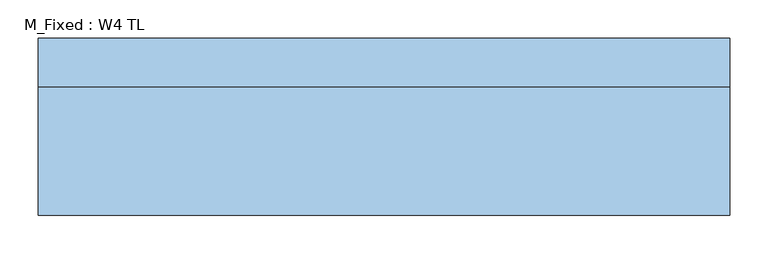
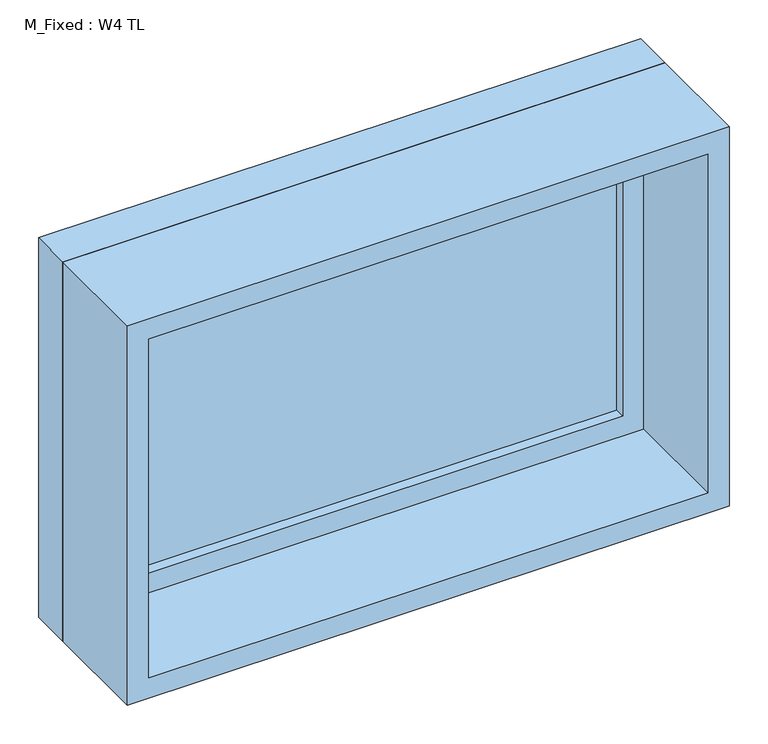
"""IFC4 building model written with IfcOpenShell, lengths in millimetres: window geometry, M_Fixed : W4 TL."""

from ifc_helpers import new_model, si_unit, frame, origin, place, context, project, spatial, polyline, outline, extrude, source, transform, mapped, element, save


def m_fixed_w4_tl_2657e552(model_context):
    return source(origin(), model_context, "Body", "SweptSolid", [
        extrude(outline(polyline([(-387.0, 93.0), (387.0, 93.0), (387.0, 81.0), (-387.0, 81.0), (-387.0, 93.0)])), frame((0.0, 0.0, 1563.0), z_axis=(0.0, 0.0, 1.0), x_axis=(1.0, 0.0, 0.0)), (0.0, 0.0, 1.0), 474.0),
        extrude(outline(polyline([(2081.0, -431.0), (1519.0, -431.0), (1519.0, 431.0), (2081.0, 431.0), (2081.0, -431.0)]), holes=[polyline([(2037.0, -387.0), (2037.0, 387.0), (1563.0, 387.0), (1563.0, -387.0), (2037.0, -387.0)])]), frame((0.0, 65.0, 0.0), z_axis=(0.0, 1.0, 0.0), x_axis=(0.0, 0.0, 1.0)), (0.0, 0.0, 1.0), 44.0),
        extrude(outline(polyline([(2100.0, -450.0), (1500.0, -450.0), (1500.0, 450.0), (2100.0, 450.0), (2100.0, -450.0)]), holes=[polyline([(2081.0, -431.0), (2081.0, 431.0), (1519.0, 431.0), (1519.0, -431.0), (2081.0, -431.0)])]), frame((0.0, 65.0, 0.0), z_axis=(0.0, 1.0, 0.0), x_axis=(0.0, 0.0, 1.0)), (0.0, 0.0, 1.0), 63.0),
        extrude(outline(polyline([(2100.0, -450.0), (1500.0, -450.0), (1500.0, 450.0), (2100.0, 450.0), (2100.0, -450.0)]), holes=[polyline([(2068.0, -418.0), (2068.0, 418.0), (1532.0, 418.0), (1532.0, -418.0), (2068.0, -418.0)])]), frame((0.0, -102.0, 0.0), z_axis=(0.0, 1.0, 0.0), x_axis=(0.0, 0.0, 1.0)), (0.0, 0.0, 1.0), 167.0),
    ])


if __name__ == "__main__":
    model = new_model("IFC4")
    model_context = context("Model", 3, world=origin())
    ifc_project = project(units=[si_unit("LENGTHUNIT", "METRE", prefix="MILLI")], contexts=[model_context])
    site = spatial("IfcSite", under=ifc_project)
    building = spatial("IfcBuilding", under=site)
    placement = place(None, origin())
    m_fixed_w4_tl_shape = m_fixed_w4_tl_2657e552(model_context)
    element("IfcWindow", 1, ObjectType="M_Fixed : W4 TL", at=placement, inside=building, context=model_context, shape_type="MappedRepresentation", body=[
        mapped(m_fixed_w4_tl_shape, transform((0.0, 0.0, 0.0), x_axis=(1.0, 0.0, 0.0), y_axis=(0.0, 1.0, 0.0), z_axis=(0.0, 0.0, 1.0))),
    ])
    save(model, "model.ifc")

# Revit data of these elements
# Type "M_Fixed : W4 TL"
#   Type Mark = "22"
#   Height = 600 mm
#   Default Sill Height = 1500 mm
#   Width = 900 mm
#   Window Inset = 19 mm
#   Frame Exterior Material = Iron, Ductile
#   Frame Interior Material = Iron, Ductile
#   Glass Pane Material = Glass
#   Sash = Iron, Ductile
#   Wall Closure = (empty or 0)
# Element 1 (IfcWindow, "M_Fixed : W4 TL")
#   Materials on its faces: "Iron, Ductile", "Glass"
# Materials
#   "Iron, Ductile": class "Metal", colour RGB 90 97 102, transparency 0, Description = "Ductile cast iron", Cost = 0
#   "Glass": class "Glass", colour RGB 218 227 224, transparency 0.85, Description = "Soda Lime Glass", Cost = 0
